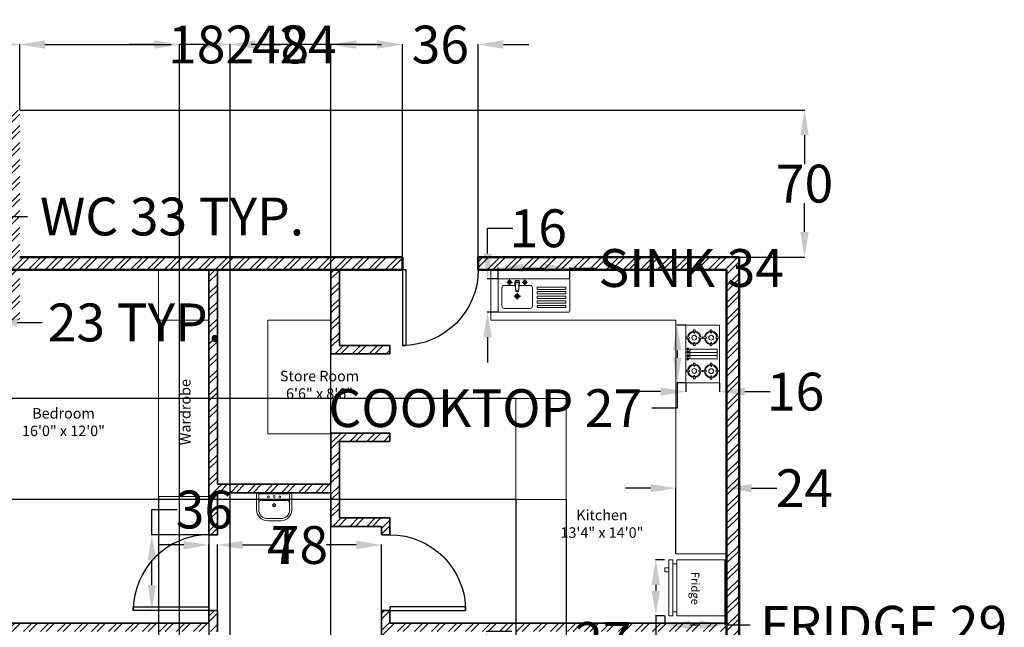
# Model space of a CAD drawing. Units: inches. Extents: x 7 to 752, y -275 to 426.
# Tile 5 of 5: x 284 to 752, y 137 to 426. Entities that reach past the tile are written whole.
import ezdxf

# ---------------------------------------------------------------- set-up
doc = ezdxf.new("R2010")
doc.units = ezdxf.units.IN
for name, color, linetype, lineweight in [('A-ANNO-DIMS', 2, 'Continuous', 18), ('A-ANNO-TEXT', 7, 'Continuous', 18), ('A-AREA-IDEN', 7, 'Continuous', 18), ('A-DOOR', 6, 'Continuous', 25), ('A-EQPM', 3, 'Continuous', 18), ('A-FLOR-CASE', 2, 'Continuous', 18), ('A-FLOR-FIXT', 8, 'Continuous', 18), ('A-WALL-PATT', 252, 'Continuous', 13), ('Inner Wall', 5, 'Continuous', 35), ('Kitchen', 3, 'Continuous', 18), ('Outer Wall', 1, 'Continuous', 50)]:
    doc.layers.add(name, color=color, linetype=linetype, lineweight=lineweight)
doc.styles.get("Standard").update_dxf_attribs({"font": 'arial.ttf'})
doc.dimstyles.get("Standard").update_dxf_attribs({"dimtxt": 18, "dimasz": 12, "dimexe": 0.18, "dimexo": 0.0625, "dimgap": 0.09, "dimtad": 0, "dimtih": 1, "dimtoh": 1, "dimdec": 0, "dimzin": 0, "dimdsep": 46, "dimlunit": 3, "dimtxsty": 'Standard', "dimcen": 0.09, "dimadec": 0, "dimazin": 0, "dimtfac": 1, "dimtdec": 0, "dimtofl": 0, "dimtmove": 0, "dimatfit": 3, "dimfxl": 1, "dimtolj": 1, "dimtzin": 0, "dimarcsym": 0})
pattern_1 = [(45, (-434.707, -1257.0093), (-4.041115, 4.041115), []), (45, (-432.013, -1257.0093), (-4.041115, 4.041115), [])]

# ---------------------------------------------------------------- blocks, each defined once
blk = doc.blocks.new('*U3')
for p, q in [((0, 0), (0, -4)), ((36, 0), (36, -4))]:
    blk.add_line(p, q)
blk.add_lwpolyline([(0, 0), (0, 36), (1.75, 36), (1.75, 0)], close=True)
blk.add_arc((0, 0), 36, 0, 90)
blk = doc.blocks.new('*U5')
for p, q in [((0, 0), (0, -6)), ((36, 0), (36, -6))]:
    blk.add_line(p, q)
blk.add_lwpolyline([(0, 0), (0, 36), (1.75, 36), (1.75, 0)], close=True)
blk.add_arc((0, 0), 36, 0, 90)
blk = doc.blocks.new('A$C7C492201')
for p, q in [((0, 10), (0, 427)), ((10, 437), (927, 437)), ((112, 389), (185, 389)), ((148, 425), (148, 352)), ((223, 415), (217, 376)), ((223, 415), (232, 268)), ((223, 415), (248, 415)), ((225, 395), (248, 395)), ((273, 415), (248, 415)), ((272, 395), (248, 395)), ((273, 415), (265, 268)), ((273, 415), (280, 376)), ((312, 389), (385, 389)), ((348, 425), (348, 352)), ((937, 10), (937, 427)), ((48, 319), (48, 79)), ((221, 349), (78, 349)), ((217, 376), (232, 268)), ((231, 279), (248, 279)), ((232, 268), (248, 268)), ((266, 279), (248, 279)), ((265, 268), (248, 268)), ((280, 376), (265, 268)), ((418, 349), (276, 349)), ((448, 319), (448, 79)), ((509, 328), (509, 298)), ((509, 328), (885, 328)), ((509, 298), (885, 298)), ((509, 268), (509, 238)), ((509, 268), (885, 268)), ((885, 328), (885, 298)), ((885, 268), (885, 238)), ((203, 208), (294, 208)), ((248, 253), (248, 163)), ((509, 238), (885, 238)), ((509, 208), (885, 208)), ((509, 208), (509, 178)), ((509, 178), (885, 178)), ((509, 148), (509, 118)), ((509, 148), (885, 148)), ((885, 208), (885, 178)), ((885, 148), (885, 118)), ((927, 0), (10, 0)), ((418, 49), (78, 49)), ((509, 118), (885, 118)), ((509, 88), (509, 58)), ((509, 88), (885, 88)), ((509, 58), (885, 58)), ((885, 88), (885, 58))]:
    blk.add_line(p, q)
for centre, radius in [((148, 389), 25), ((148, 389), 15), ((348, 389), 25), ((348, 389), 15), ((248, 208), 30), ((248, 208), 20)]:
    blk.add_circle(centre, radius)
for centre, radius, start, end in [((10, 427), 10, 90, 180), ((247, 388), 7.19, 80.5252, 279.4748), ((250, 388), 7.19, 260.5252, 99.4748), ((927, 427), 10, 0, 90), ((78, 319), 30, 90, 180), ((418, 319), 30, 0, 90), ((10, 10), 10, 180, 270), ((78, 79), 30, 180, 270), ((418, 79), 30, 270, 0), ((927, 10), 10, 270, 0)]:
    blk.add_arc(centre, radius, start, end)
blk = doc.blocks.new('REFRI-00')
for points in [[(-0.35, 0.35), (-0.35, -0.25), (0.35, -0.25), (0.35, 0.35), (-0.35, 0.35)], [(-0.35, -0.3), (-0.35, -0.35), (0.35, -0.35), (0.35, -0.3), (-0.35, -0.3)], [(-0.3, -0.3), (-0.3, -0.25)], [(-0.25, -0.35), (-0.25, -0.4), (-0.2, -0.4), (-0.2, -0.35)], [(0.3, -0.3), (0.3, -0.25)]]:
    blk.add_lwpolyline(points)
blk = doc.blocks.new('A$C57CF26DA')
for p, q in [((0, 0), (0, 420)), ((720, 420), (0, 420)), ((167, 413), (147, 413)), ((147, 413), (152, 373)), ((152, 373), (162, 373)), ((162, 373), (167, 413)), ((300, 391), (300, 49)), ((300, 391), (420, 391)), ((340, 391), (340, 49)), ((380, 391), (380, 49)), ((420, 391), (420, 49)), ((584, 413), (564, 413)), ((564, 413), (569, 373)), ((569, 373), (579, 373)), ((579, 373), (584, 413)), ((720, 0), (720, 420)), ((99, 320), (59, 325)), ((59, 325), (59, 305)), ((59, 305), (99, 310)), ((99, 310), (99, 320)), ((152, 257), (147, 217)), ((162, 257), (152, 257)), ((167, 217), (162, 257)), ((255, 325), (215, 320)), ((215, 320), (215, 310)), ((215, 310), (255, 305)), ((255, 305), (255, 325)), ((516, 320), (476, 325)), ((476, 325), (476, 305)), ((476, 305), (516, 310)), ((516, 310), (516, 320)), ((569, 257), (564, 217)), ((579, 257), (569, 257)), ((584, 217), (579, 257)), ((672, 325), (632, 320)), ((632, 320), (632, 310)), ((632, 310), (672, 305)), ((672, 305), (672, 325)), ((147, 217), (167, 217)), ((167, 203), (147, 203)), ((147, 203), (152, 163)), ((152, 163), (162, 163)), ((162, 163), (167, 203)), ((581, 203), (561, 203)), ((561, 203), (566, 163)), ((564, 217), (584, 217)), ((566, 163), (576, 163)), ((576, 163), (581, 203)), ((99, 110), (59, 115)), ((59, 115), (59, 95)), ((59, 95), (99, 100)), ((99, 100), (99, 110)), ((152, 47), (147, 7)), ((147, 7), (167, 7)), ((162, 47), (152, 47)), ((167, 7), (162, 47)), ((255, 115), (215, 110)), ((215, 110), (215, 100)), ((215, 100), (255, 95)), ((255, 95), (255, 115)), ((302, 39), (295, 39)), ((295, 39), (295, 11)), ((295, 11), (302, 11)), ((420, 49), (300, 49)), ((302, 11), (302, 39)), ((341, 39), (334, 39)), ((334, 39), (334, 11)), ((334, 11), (341, 11)), ((341, 11), (341, 39)), ((380, 11), (380, 39)), ((380, 39), (386, 39)), ((386, 11), (380, 11)), ((386, 39), (386, 11)), ((419, 11), (419, 39)), ((419, 39), (426, 39)), ((426, 11), (419, 11)), ((426, 39), (426, 11)), ((513, 110), (473, 115)), ((473, 115), (473, 95)), ((473, 95), (513, 100)), ((513, 100), (513, 110)), ((566, 47), (561, 7)), ((561, 7), (581, 7)), ((576, 47), (566, 47)), ((581, 7), (576, 47)), ((669, 115), (629, 110)), ((629, 110), (629, 100)), ((629, 100), (669, 95)), ((669, 95), (669, 115)), ((720, 0), (0, 0))]:
    blk.add_line(p, q)
for centre in [(157, 315), (574, 315), (157, 105), (571, 105)]:
    blk.add_circle(centre, 30)
for centre, radius, start, end in [((157, 315), 83, 95.5849, 174.4151), ((157, 315), 73, 95.3738, 174.6262), ((157, 315), 73, 5.3738, 84.6262), ((157, 315), 83, 5.5849, 84.4151), ((574, 315), 83, 95.5849, 174.4151), ((574, 315), 73, 95.3738, 174.6262), ((574, 315), 73, 5.3738, 84.6262), ((574, 315), 83, 5.5849, 84.4151), ((157, 315), 83, 185.5849, 264.4151), ((157, 315), 73, 185.3738, 264.6262), ((157, 315), 73, 275.3738, 354.6262), ((157, 315), 83, 275.5849, 354.4151), ((574, 315), 83, 185.5849, 264.4151), ((574, 315), 73, 185.3738, 264.6262), ((574, 315), 73, 275.3738, 354.6262), ((574, 315), 83, 275.5849, 354.4151), ((157, 105), 83, 95.5849, 174.4151), ((157, 105), 73, 95.3738, 174.6262), ((157, 105), 73, 5.3738, 84.6262), ((157, 105), 83, 5.5849, 84.4151), ((571, 105), 83, 95.5849, 174.4151), ((571, 105), 73, 95.3738, 174.6262), ((571, 105), 73, 5.3738, 84.6262), ((571, 105), 83, 5.5849, 84.4151), ((157, 105), 83, 185.5849, 264.4151), ((157, 105), 73, 185.3738, 264.6262), ((157, 105), 73, 275.3738, 354.6262), ((157, 105), 83, 275.5849, 354.4151), ((298, 25), 13.7, 104.4775, 255.5225), ((298, 25), 13.7, 284.4775, 75.5225), ((337, 25), 13.7, 104.4775, 255.5225), ((337, 25), 13.7, 284.4775, 75.5225), ((383, 25), 13.7, 104.4775, 255.5225), ((383, 25), 13.7, 284.4775, 75.5225), ((422, 25), 13.7, 104.4775, 255.5225), ((422, 25), 13.7, 284.4775, 75.5225), ((571, 105), 83, 185.5849, 264.4151), ((571, 105), 73, 185.3738, 264.6262), ((571, 105), 73, 275.3738, 354.6262), ((571, 105), 83, 275.5849, 354.4151)]:
    blk.add_arc(centre, radius, start, end)
blk = doc.blocks.new('A$C57EA129C')
for p, q in [((0, 0.443), (0, 0.178)), ((0.016, 0.459), (0.563, 0.459)), ((0.036, 0.432), (0.036, 0.29)), ((0.045, 0.441), (0.535, 0.441)), ((0.08, 0.334), (0.499, 0.334)), ((0.544, 0.432), (0.544, 0.29)), ((0.579, 0.443), (0.579, 0.178)), ((0.036, 0.29), (0.036, 0.178)), ((0.544, 0.29), (0.544, 0.178)), ((0.178, 0.036), (0.401, 0.036)), ((0.178, 0), (0.401, 0))]:
    blk.add_line(p, q)
for centre, radius in [((0.198, 0.392), 0.0143), ((0.29, 0.396), 0.0156), ((0.381, 0.392), 0.0143), ((0.29, 0.255), 0.0267), ((0.29, 0.255), 0.0178)]:
    blk.add_circle(centre, radius)
for centre, radius, start, end in [((0.016, 0.443), 0.016, 90, 180), ((0.045, 0.432), 0.00891, 90, 180), ((0.08, 0.29), 0.0445, 90, 180), ((0.499, 0.29), 0.0445, 0, 90), ((0.535, 0.432), 0.00891, 0, 90), ((0.563, 0.443), 0.016, 0, 90), ((0.178, 0.178), 0.178, 180, 270), ((0.178, 0.178), 0.143, 180, 270), ((0.401, 0.178), 0.178, 270, 0), ((0.401, 0.178), 0.143, 270, 0)]:
    blk.add_arc(centre, radius, start, end)
blk = doc.blocks.new('*D16')
at = {"layer": 'A-ANNO-DIMS', "color": 0, "lineweight": -2, "transparency": 16777216}
for p, q in [((276.06, 320.03), (276.06, 332.03)), ((276.06, 332.03), (288.06, 332.03)), ((271.12, 320.03), (276.24, 320.03)), ((276.06, 298.68), (276.06, 308.03)), ((271.12, 286.68), (276.24, 286.68))]:
    blk.add_line(p, q, dxfattribs=at)
at = {"layer": 'A-ANNO-DIMS', "color": 0, "transparency": 16777216}
for points in [[(274.06, 308.03), (278.06, 308.03), (276.06, 320.03)], [(274.06, 298.68), (278.06, 298.68), (276.06, 286.68)]]:
    blk.add_solid(points, dxfattribs=at)
at = {"layer": 'Defpoints', "color": 0, "transparency": 16777216}
for p in [(271.06, 320.03), (276.06, 320.03), (271.06, 286.68)]:
    blk.add_point(p, dxfattribs=at)
at = {"layer": 'A-ANNO-DIMS', "color": 0, "transparency": 16777216, "insert": (356.77, 332.03), "char_height": 18, "attachment_point": 5}
blk.add_mtext('\\A1;WC 33 TYP.', dxfattribs=at)
blk = doc.blocks.new('*D17')
at = {"layer": 'A-ANNO-DIMS', "color": 0, "lineweight": -2, "transparency": 16777216}
for p, q in [((247.6, 286.61), (247.6, 281.49)), ((271.06, 286.61), (271.06, 281.49)), ((235.6, 281.67), (223.6, 281.67)), ((283.06, 281.67), (295.06, 281.67))]:
    blk.add_line(p, q, dxfattribs=at)
at = {"layer": 'A-ANNO-DIMS', "color": 0, "transparency": 16777216}
for points in [[(235.6, 283.67), (235.6, 279.67), (247.6, 281.67)], [(283.06, 283.67), (283.06, 279.67), (271.06, 281.67)]]:
    blk.add_solid(points, dxfattribs=at)
at = {"layer": 'Defpoints', "color": 0, "transparency": 16777216}
for p in [(247.6, 286.68), (271.06, 286.68), (271.06, 281.67)]:
    blk.add_point(p, dxfattribs=at)
at = {"layer": 'A-ANNO-DIMS', "color": 0, "transparency": 16777216, "insert": (339.11, 281.67), "char_height": 18, "attachment_point": 5}
blk.add_mtext('\\A1;23 TYP.', dxfattribs=at)
blk = doc.blocks.new('*D20')
at = {"layer": 'A-ANNO-DIMS', "color": 0, "lineweight": -2, "transparency": 16777216}
for p, q in [((518.33, 134.68), (506.15, 134.68)), ((506.33, 122.68), (506.33, 103.84)), ((506.33, 66.2), (506.33, 85.04)), ((518.33, 54.2), (506.15, 54.2))]:
    blk.add_line(p, q, dxfattribs=at)
at = {"layer": 'A-ANNO-DIMS', "color": 0, "transparency": 16777216}
for points in [[(504.33, 122.68), (508.33, 122.68), (506.33, 134.68)], [(504.33, 66.2), (508.33, 66.2), (506.33, 54.2)]]:
    blk.add_solid(points, dxfattribs=at)
at = {"layer": 'Defpoints', "color": 0, "transparency": 16777216}
for p in [(506.33, 134.68), (518.4, 134.68), (518.4, 54.2)]:
    blk.add_point(p, dxfattribs=at)
at = {"layer": 'A-ANNO-DIMS', "color": 0, "transparency": 16777216, "insert": (506.33, 94.44), "char_height": 18, "attachment_point": 5}
blk.add_mtext('\\A1;KING BED 80 TYP.', dxfattribs=at)
blk = doc.blocks.new('*D24')
at = {"layer": 'A-ANNO-DIMS', "color": 0, "lineweight": -2, "transparency": 16777216}
for p, q in [((511.85, 302.5), (511.85, 307.72)), ((523.85, 307.54), (533.86, 307.54)), ((545.86, 302.5), (545.86, 307.72)), ((545.86, 307.54), (557.86, 307.54))]:
    blk.add_line(p, q, dxfattribs=at)
at = {"layer": 'A-ANNO-DIMS', "color": 0, "transparency": 16777216}
for points in [[(523.85, 309.54), (523.85, 305.54), (511.85, 307.54)], [(533.86, 309.54), (533.86, 305.54), (545.86, 307.54)]]:
    blk.add_solid(points, dxfattribs=at)
at = {"layer": 'Defpoints', "color": 0, "transparency": 16777216}
for p in [(545.86, 307.54), (511.85, 302.44), (545.86, 302.44)]:
    blk.add_point(p, dxfattribs=at)
at = {"layer": 'A-ANNO-DIMS', "color": 0, "transparency": 16777216, "insert": (603.6, 307.54), "char_height": 18, "attachment_point": 5}
blk.add_mtext('\\A1;SINK 34', dxfattribs=at)
blk = doc.blocks.new('*D25')
at = {"layer": 'A-ANNO-DIMS', "color": 0, "lineweight": -2, "transparency": 16777216}
for p, q in [((506.75, 314.44), (506.75, 326.44)), ((506.75, 326.44), (518.75, 326.44)), ((511.79, 302.44), (506.57, 302.44)), ((511.79, 286.59), (506.57, 286.59)), ((506.75, 274.59), (506.75, 262.59))]:
    blk.add_line(p, q, dxfattribs=at)
at = {"layer": 'A-ANNO-DIMS', "color": 0, "transparency": 16777216}
for points in [[(504.75, 314.44), (508.75, 314.44), (506.75, 302.44)], [(504.75, 274.59), (508.75, 274.59), (506.75, 286.59)]]:
    blk.add_solid(points, dxfattribs=at)
at = {"layer": 'Defpoints', "color": 0, "transparency": 16777216}
for p in [(506.75, 302.44), (511.85, 302.44), (511.85, 286.59)]:
    blk.add_point(p, dxfattribs=at)
at = {"layer": 'A-ANNO-DIMS', "color": 0, "transparency": 16777216, "insert": (530.88, 326.44), "char_height": 18, "attachment_point": 5}
blk.add_mtext('\\A1;16', dxfattribs=at)
blk = doc.blocks.new('*D26')
at = {"layer": 'A-ANNO-DIMS', "color": 0, "lineweight": -2, "transparency": 16777216}
for p, q in [((591.04, 142.1), (591.04, 137.69)), ((619.61, 142.1), (619.61, 137.69)), ((603.04, 137.87), (607.61, 137.87)), ((619.61, 137.87), (631.61, 137.87))]:
    blk.add_line(p, q, dxfattribs=at)
at = {"layer": 'A-ANNO-DIMS', "color": 0, "transparency": 16777216}
for points in [[(603.04, 139.87), (603.04, 135.87), (591.04, 137.87)], [(607.61, 139.87), (607.61, 135.87), (619.61, 137.87)]]:
    blk.add_solid(points, dxfattribs=at)
at = {"layer": 'Defpoints', "color": 0, "transparency": 16777216}
for p in [(591.04, 142.16), (619.61, 142.16), (619.61, 137.87)]:
    blk.add_point(p, dxfattribs=at)
at = {"layer": 'A-ANNO-DIMS', "color": 0, "transparency": 16777216, "insert": (695.1, 137.87), "char_height": 18, "attachment_point": 5}
blk.add_mtext('\\A1;FRIDGE 29', dxfattribs=at)
blk = doc.blocks.new('*D27')
at = {"layer": 'A-ANNO-DIMS', "color": 0, "lineweight": -2, "transparency": 16777216}
for p, q in [((590.98, 168.83), (586.58, 168.83)), ((586.76, 156.83), (586.76, 154.16)), ((590.98, 142.16), (586.58, 142.16)), ((586.76, 142.16), (586.76, 130.16)), ((586.76, 130.16), (574.76, 130.16))]:
    blk.add_line(p, q, dxfattribs=at)
at = {"layer": 'A-ANNO-DIMS', "color": 0, "transparency": 16777216}
for points in [[(584.76, 156.83), (588.76, 156.83), (586.76, 168.83)], [(584.76, 154.16), (588.76, 154.16), (586.76, 142.16)]]:
    blk.add_solid(points, dxfattribs=at)
at = {"layer": 'Defpoints', "color": 0, "transparency": 16777216}
for p in [(591.04, 168.83), (586.76, 142.16), (591.04, 142.16)]:
    blk.add_point(p, dxfattribs=at)
at = {"layer": 'A-ANNO-DIMS', "color": 0, "transparency": 16777216, "insert": (561.62, 130.16), "char_height": 18, "attachment_point": 5}
blk.add_mtext('\\A1;27', dxfattribs=at)
blk = doc.blocks.new('*D28')
at = {"layer": 'A-ANNO-DIMS', "color": 0, "lineweight": -2, "transparency": 16777216}
for p, q in [((600.98, 280.39), (596.74, 280.39)), ((596.92, 268.39), (596.92, 264.9)), ((600.98, 252.9), (596.74, 252.9)), ((596.92, 252.9), (596.92, 240.9)), ((596.92, 240.9), (584.92, 240.9))]:
    blk.add_line(p, q, dxfattribs=at)
at = {"layer": 'A-ANNO-DIMS', "color": 0, "transparency": 16777216}
for points in [[(594.92, 268.39), (598.92, 268.39), (596.92, 280.39)], [(594.92, 264.9), (598.92, 264.9), (596.92, 252.9)]]:
    blk.add_solid(points, dxfattribs=at)
at = {"layer": 'Defpoints', "color": 0, "transparency": 16777216}
for p in [(601.05, 280.39), (596.92, 252.9), (601.05, 252.9)]:
    blk.add_point(p, dxfattribs=at)
at = {"layer": 'A-ANNO-DIMS', "color": 0, "transparency": 16777216, "insert": (505.68, 240.9), "char_height": 18, "attachment_point": 5}
blk.add_mtext('\\A1;COOKTOP 27', dxfattribs=at)
blk = doc.blocks.new('*D29')
at = {"layer": 'A-ANNO-DIMS', "color": 0, "lineweight": -2, "transparency": 16777216}
for p, q in [((601.05, 252.84), (601.05, 248.6)), ((617.08, 252.84), (617.08, 248.6)), ((589.05, 248.78), (577.05, 248.78)), ((629.08, 248.78), (641.08, 248.78))]:
    blk.add_line(p, q, dxfattribs=at)
at = {"layer": 'A-ANNO-DIMS', "color": 0, "transparency": 16777216}
for points in [[(589.05, 250.78), (589.05, 246.78), (601.05, 248.78)], [(629.08, 250.78), (629.08, 246.78), (617.08, 248.78)]]:
    blk.add_solid(points, dxfattribs=at)
at = {"layer": 'Defpoints', "color": 0, "transparency": 16777216}
for p in [(601.05, 252.9), (617.08, 252.9), (617.08, 248.78)]:
    blk.add_point(p, dxfattribs=at)
at = {"layer": 'A-ANNO-DIMS', "color": 0, "transparency": 16777216, "insert": (653.21, 248.78), "char_height": 18, "attachment_point": 5}
blk.add_mtext('\\A1;16', dxfattribs=at)
blk = doc.blocks.new('*D33')
at = {"layer": 'A-ANNO-DIMS', "color": 0, "lineweight": -2, "transparency": 16777216}
for p, q in [((176.33, 382.74), (176.33, 414.01)), ((188.33, 413.83), (211.18, 413.83)), ((272.33, 413.83), (249.47, 413.83)), ((284.33, 382.74), (284.33, 414.01))]:
    blk.add_line(p, q, dxfattribs=at)
at = {"layer": 'A-ANNO-DIMS', "color": 0, "transparency": 16777216}
for points in [[(188.33, 415.83), (188.33, 411.83), (176.33, 413.83)], [(272.33, 415.83), (272.33, 411.83), (284.33, 413.83)]]:
    blk.add_solid(points, dxfattribs=at)
at = {"layer": 'Defpoints', "color": 0, "transparency": 16777216}
for p in [(284.33, 413.83), (176.33, 382.68), (284.33, 382.68)]:
    blk.add_point(p, dxfattribs=at)
at = {"layer": 'A-ANNO-DIMS', "color": 0, "transparency": 16777216, "insert": (230.33, 413.83), "char_height": 18, "attachment_point": 5}
blk.add_mtext('\\A1;108', dxfattribs=at)
blk = doc.blocks.new('*D34')
at = {"layer": 'A-ANNO-DIMS', "color": 0, "lineweight": -2, "transparency": 16777216}
for p, q in [((284.33, 382.74), (284.33, 414.01)), ((296.33, 413.83), (356.29, 413.83)), ((454.33, 413.83), (394.36, 413.83)), ((466.33, 312.74), (466.33, 414.01))]:
    blk.add_line(p, q, dxfattribs=at)
at = {"layer": 'A-ANNO-DIMS', "color": 0, "transparency": 16777216}
for points in [[(296.33, 415.83), (296.33, 411.83), (284.33, 413.83)], [(454.33, 415.83), (454.33, 411.83), (466.33, 413.83)]]:
    blk.add_solid(points, dxfattribs=at)
at = {"layer": 'Defpoints', "color": 0, "transparency": 16777216}
for p in [(466.33, 413.83), (284.33, 382.68), (466.33, 312.68)]:
    blk.add_point(p, dxfattribs=at)
at = {"layer": 'A-ANNO-DIMS', "color": 0, "transparency": 16777216, "insert": (375.33, 413.83), "char_height": 18, "attachment_point": 5}
blk.add_mtext('\\A1;182', dxfattribs=at)
blk = doc.blocks.new('*D35')
at = {"layer": 'A-ANNO-DIMS', "color": 0, "lineweight": -2, "transparency": 16777216}
for p, q in [((454.328243, 413.826615), (442.328243, 413.826615)), ((466.328243, 312.739115), (466.328243, 414.006615)), ((502.328243, 312.739115), (502.328243, 414.006615)), ((514.328243, 413.826615), (526.328243, 413.826615))]:
    blk.add_line(p, q, dxfattribs=at)
at = {"layer": 'A-ANNO-DIMS', "color": 0, "transparency": 16777216}
for points in [[(454.328243, 415.826615), (454.328243, 411.826615), (466.328243, 413.826615)], [(514.328243, 415.826615), (514.328243, 411.826615), (502.328243, 413.826615)]]:
    blk.add_solid(points, dxfattribs=at)
at = {"layer": 'Defpoints', "color": 0, "transparency": 16777216}
for p in [(502.328243, 413.826615), (466.328243, 312.676615), (502.328243, 312.676615)]:
    blk.add_point(p, dxfattribs=at)
at = {"layer": 'A-ANNO-DIMS', "color": 0, "transparency": 16777216, "insert": (484.328243, 413.826615), "char_height": 18, "attachment_point": 5}
blk.add_mtext('\\A1;36', dxfattribs=at)
blk = doc.blocks.new('*D36')
at = {"layer": 'A-ANNO-DIMS', "color": 0, "lineweight": -2, "transparency": 16777216}
for p, q in [((284.39, 382.68), (657.66, 382.68)), ((657.48, 370.68), (657.48, 356.96)), ((657.48, 324.68), (657.48, 338.4)), ((626.39, 312.68), (657.66, 312.68))]:
    blk.add_line(p, q, dxfattribs=at)
at = {"layer": 'A-ANNO-DIMS', "color": 0, "transparency": 16777216}
for points in [[(655.48, 370.68), (659.48, 370.68), (657.48, 382.68)], [(655.48, 324.68), (659.48, 324.68), (657.48, 312.68)]]:
    blk.add_solid(points, dxfattribs=at)
at = {"layer": 'Defpoints', "color": 0, "transparency": 16777216}
for p in [(284.33, 382.68), (626.33, 312.68), (657.48, 312.68)]:
    blk.add_point(p, dxfattribs=at)
at = {"layer": 'A-ANNO-DIMS', "color": 0, "transparency": 16777216, "insert": (657.48, 347.68), "char_height": 18, "attachment_point": 5}
blk.add_mtext('\\A1;70', dxfattribs=at)
blk = doc.blocks.new('*D39')
at = {"layer": 'A-ANNO-DIMS', "color": 0, "lineweight": -2, "transparency": 16777216}
for p, q in [((348.33, 413.83), (336.33, 413.83)), ((360.33, -131.26), (360.33, 414.01)), ((384.33, -131.26), (384.33, 414.01)), ((396.33, 413.83), (408.33, 413.83))]:
    blk.add_line(p, q, dxfattribs=at)
at = {"layer": 'A-ANNO-DIMS', "color": 0, "transparency": 16777216}
for points in [[(348.33, 415.83), (348.33, 411.83), (360.33, 413.83)], [(396.33, 415.83), (396.33, 411.83), (384.33, 413.83)]]:
    blk.add_solid(points, dxfattribs=at)
at = {"layer": 'Defpoints', "color": 0, "transparency": 16777216}
for p in [(384.33, 413.83), (360.33, -131.32), (384.33, -131.32)]:
    blk.add_point(p, dxfattribs=at)
at = {"layer": 'A-ANNO-DIMS', "color": 0, "transparency": 16777216, "insert": (421.43, 413.83), "char_height": 18, "attachment_point": 5}
blk.add_mtext('\\A1;24', dxfattribs=at)
blk = doc.blocks.new('*D40')
at = {"layer": 'A-ANNO-DIMS', "color": 0, "lineweight": -2, "transparency": 16777216}
for p, q in [((372.328243, 413.826615), (360.328243, 413.826615)), ((384.328243, -106.961989), (384.328243, 414.006615)), ((432.328243, -106.961989), (432.328243, 414.006615)), ((444.328243, 413.826615), (456.328243, 413.826615))]:
    blk.add_line(p, q, dxfattribs=at)
at = {"layer": 'A-ANNO-DIMS', "color": 0, "transparency": 16777216}
for points in [[(372.328243, 415.826615), (372.328243, 411.826615), (384.328243, 413.826615)], [(444.328243, 415.826615), (444.328243, 411.826615), (432.328243, 413.826615)]]:
    blk.add_solid(points, dxfattribs=at)
at = {"layer": 'Defpoints', "color": 0, "transparency": 16777216}
for p in [(432.328243, 413.826615), (384.328243, -107.024489), (432.328243, -107.024489)]:
    blk.add_point(p, dxfattribs=at)
at = {"layer": 'A-ANNO-DIMS', "color": 0, "transparency": 16777216, "insert": (408.328243, 413.826615), "char_height": 18, "attachment_point": 5}
blk.add_mtext('\\A1;48', dxfattribs=at)
blk = doc.blocks.new('*D46')
at = {"layer": 'A-ANNO-DIMS', "color": 0, "lineweight": -2, "transparency": 16777216}
for p, q in [((520.16, 197.44), (520.16, -259.65)), ((544.16, 197.44), (544.16, -259.65)), ((508.16, -259.47), (496.16, -259.47)), ((556.16, -259.47), (568.16, -259.47))]:
    blk.add_line(p, q, dxfattribs=at)
at = {"layer": 'A-ANNO-DIMS', "color": 0, "transparency": 16777216}
for points in [[(508.16, -257.47), (508.16, -261.47), (520.16, -259.47)], [(556.16, -257.47), (556.16, -261.47), (544.16, -259.47)]]:
    blk.add_solid(points, dxfattribs=at)
at = {"layer": 'Defpoints', "color": 0, "transparency": 16777216}
for p in [(520.16, 197.5), (544.16, 197.5), (544.16, -259.47)]:
    blk.add_point(p, dxfattribs=at)
at = {"layer": 'A-ANNO-DIMS', "color": 0, "transparency": 16777216, "insert": (581.26, -259.47), "char_height": 18, "attachment_point": 5}
blk.add_mtext('\\A1;24', dxfattribs=at)
blk = doc.blocks.new('*D47')
at = {"layer": 'A-ANNO-DIMS', "color": 0, "lineweight": -2, "transparency": 16777216}
for p, q in [((520.1, 245.5), (127, 245.5)), ((127.18, 233.5), (127.18, 230.78)), ((127.18, 209.5), (127.18, 212.22)), ((520.1, 197.5), (127, 197.5))]:
    blk.add_line(p, q, dxfattribs=at)
at = {"layer": 'A-ANNO-DIMS', "color": 0, "transparency": 16777216}
for points in [[(125.18, 233.5), (129.18, 233.5), (127.18, 245.5)], [(125.18, 209.5), (129.18, 209.5), (127.18, 197.5)]]:
    blk.add_solid(points, dxfattribs=at)
at = {"layer": 'Defpoints', "color": 0, "transparency": 16777216}
for p in [(127.18, 245.5), (520.16, 245.5), (520.16, 197.5)]:
    blk.add_point(p, dxfattribs=at)
at = {"layer": 'A-ANNO-DIMS', "color": 0, "transparency": 16777216, "insert": (127.18, 221.5), "char_height": 18, "attachment_point": 5}
blk.add_mtext('\\A1;48', dxfattribs=at)
blk = doc.blocks.new('*D48')
at = {"layer": 'A-ANNO-DIMS', "color": 0, "lineweight": -2, "transparency": 16777216}
for p, q in [((584.33, 202.83), (572.33, 202.83)), ((596.33, 171.74), (596.33, 203.01)), ((620.33, 171.74), (620.33, 203.01)), ((632.33, 202.83), (644.33, 202.83))]:
    blk.add_line(p, q, dxfattribs=at)
at = {"layer": 'A-ANNO-DIMS', "color": 0, "transparency": 16777216}
for points in [[(584.33, 204.83), (584.33, 200.83), (596.33, 202.83)], [(632.33, 204.83), (632.33, 200.83), (620.33, 202.83)]]:
    blk.add_solid(points, dxfattribs=at)
at = {"layer": 'Defpoints', "color": 0, "transparency": 16777216}
for p in [(620.33, 202.83), (596.33, 171.68), (620.33, 171.68)]:
    blk.add_point(p, dxfattribs=at)
at = {"layer": 'A-ANNO-DIMS', "color": 0, "transparency": 16777216, "insert": (657.43, 202.83), "char_height": 18, "attachment_point": 5}
blk.add_mtext('\\A1;24', dxfattribs=at)
blk = doc.blocks.new('*D50')
at = {"layer": 'A-ANNO-DIMS', "color": 0, "lineweight": -2, "transparency": 16777216}
for p, q in [((362.33, 175.83), (350.33, 175.83)), ((374.33, 144.74), (374.33, 176.01)), ((378.33, 144.74), (378.33, 176.01)), ((390.33, 175.83), (402.33, 175.83))]:
    blk.add_line(p, q, dxfattribs=at)
at = {"layer": 'A-ANNO-DIMS', "color": 0, "transparency": 16777216}
for points in [[(362.33, 177.83), (362.33, 173.83), (374.33, 175.83)], [(390.33, 177.83), (390.33, 173.83), (378.33, 175.83)]]:
    blk.add_solid(points, dxfattribs=at)
at = {"layer": 'Defpoints', "color": 0, "transparency": 16777216}
for p in [(378.33, 175.83), (374.33, 144.68), (378.33, 144.68)]:
    blk.add_point(p, dxfattribs=at)
at = {"layer": 'A-ANNO-DIMS', "color": 0, "transparency": 16777216, "insert": (408.64, 175.83), "char_height": 18, "attachment_point": 5}
blk.add_mtext('\\A1;4', dxfattribs=at)
blk = doc.blocks.new('*D52')
at = {"layer": 'A-ANNO-DIMS', "color": 0, "lineweight": -2, "transparency": 16777216}
for p, q in [((350.33, 198.78), (350.33, -259.65)), ((374.33, 198.78), (374.33, -259.65)), ((338.33, -259.47), (326.33, -259.47)), ((386.33, -259.47), (398.33, -259.47))]:
    blk.add_line(p, q, dxfattribs=at)
at = {"layer": 'A-ANNO-DIMS', "color": 0, "transparency": 16777216}
for points in [[(338.33, -257.47), (338.33, -261.47), (350.33, -259.47)], [(386.33, -257.47), (386.33, -261.47), (374.33, -259.47)]]:
    blk.add_solid(points, dxfattribs=at)
at = {"layer": 'Defpoints', "color": 0, "transparency": 16777216}
for p in [(350.33, 198.85), (374.33, 198.85), (374.33, -259.47)]:
    blk.add_point(p, dxfattribs=at)
at = {"layer": 'A-ANNO-DIMS', "color": 0, "transparency": 16777216, "insert": (411.43, -259.47), "char_height": 18, "attachment_point": 5}
blk.add_mtext('\\A1;24', dxfattribs=at)
blk = doc.blocks.new('*D53')
at = {"layer": 'A-ANNO-DIMS', "color": 0, "lineweight": -2, "transparency": 16777216}
for p, q in [((378.33, 144.74), (378.33, 176.01)), ((390.33, 175.83), (404.4, 175.83)), ((444.33, 175.83), (430.26, 175.83)), ((456.33, 144.74), (456.33, 176.01))]:
    blk.add_line(p, q, dxfattribs=at)
at = {"layer": 'A-ANNO-DIMS', "color": 0, "transparency": 16777216}
for points in [[(390.33, 177.83), (390.33, 173.83), (378.33, 175.83)], [(444.33, 177.83), (444.33, 173.83), (456.33, 175.83)]]:
    blk.add_solid(points, dxfattribs=at)
at = {"layer": 'Defpoints', "color": 0, "transparency": 16777216}
for p in [(456.33, 175.83), (378.33, 144.68), (456.33, 144.68)]:
    blk.add_point(p, dxfattribs=at)
at = {"layer": 'A-ANNO-DIMS', "color": 0, "transparency": 16777216, "insert": (417.33, 175.83), "char_height": 18, "attachment_point": 5}
blk.add_mtext('\\A1;78', dxfattribs=at)
blk = doc.blocks.new('*D54')
at = {"layer": 'A-ANNO-DIMS', "color": 0, "lineweight": -2, "transparency": 16777216}
for p, q in [((347.18, 180.68), (347.18, 192.68)), ((347.18, 192.68), (359.18, 192.68)), ((378.27, 180.68), (347, 180.68)), ((347.18, 156.68), (347.18, 168.68)), ((378.27, 144.68), (347, 144.68))]:
    blk.add_line(p, q, dxfattribs=at)
at = {"layer": 'A-ANNO-DIMS', "color": 0, "transparency": 16777216}
for points in [[(345.18, 168.68), (349.18, 168.68), (347.18, 180.68)], [(345.18, 156.68), (349.18, 156.68), (347.18, 144.68)]]:
    blk.add_solid(points, dxfattribs=at)
at = {"layer": 'Defpoints', "color": 0, "transparency": 16777216}
for p in [(347.18, 180.68), (378.33, 180.68), (378.33, 144.68)]:
    blk.add_point(p, dxfattribs=at)
at = {"layer": 'A-ANNO-DIMS', "color": 0, "transparency": 16777216, "insert": (372.15, 192.68), "char_height": 18, "attachment_point": 5}
blk.add_mtext('\\A1;36', dxfattribs=at)

msp = doc.modelspace()

# ---------------------------------------------------------------- hatches: boundary and pattern name
at = {"layer": 'A-WALL-PATT'}
h = msp.add_hatch(dxfattribs=at)
h.set_pattern_fill('ANSI32', color=256, scale=0.6)
h.set_pattern_definition(pattern_1)
h.paths.add_polyline_path([(182.33, 376.68), (278.33, 376.68), (278.33, 306.68), (466.33, 306.68), (466.33, 312.68), (284.33, 312.68), (284.33, 382.68), (176.33, 382.68), (176.33, -48.32), (158.33, -48.32), (158.33, -228.32), (360.33, -228.32), (360.33, -137.32), (384.33, -137.32), (384.33, -131.32), (356.33, -131.32), (356.33, -222.32), (164.33, -222.32), (164.33, -54.32), (182.33, -54.32)])
h.paths.add_polyline_path([(626.33, 312.68), (502.33, 312.68), (502.33, 306.68), (620.33, 306.68), (620.33, 171.68), (620.33, -48.32), (544.33, -48.32), (544.33, -131.32), (432.33, -131.32), (432.33, -137.32), (550.33, -137.32), (550.33, -52.32), (626.33, -52.32)])
h = msp.add_hatch(dxfattribs=at)
h.set_pattern_fill('ANSI32', color=256, scale=0.6)
h.set_pattern_definition(pattern_1)
h.paths.add_polyline_path([(360.33, -48.32), (282.33, -48.32), (282.33, -44.32), (278.33, -44.32), (278.33, -48.32), (182.33, -48.32), (182.33, -54.32), (356.33, -54.32), (356.33, -89.32), (360.33, -89.32)])
h.paths.add_polyline_path([(484.33, -48.32), (460.33, -48.32), (460.33, -42.32), (456.33, -42.32), (456.33, -48.32), (432.33, -48.32), (432.33, -52.32), (456.33, -52.32), (456.33, -131.32), (460.33, -131.32), (460.33, -52.32), (484.33, -52.32)])
h.paths.add_polyline_path([(544.33, -48.32), (512.33, -48.32), (512.33, -52.32), (544.33, -52.32)])
h.paths.add_polyline_path([(460.33, 134.68), (484.33, 134.68), (620.33, 134.68), (620.33, 138.68), (460.33, 138.68), (460.33, 144.68), (456.33, 144.68), (456.33, -6.32), (460.33, -6.32)])
h.paths.add_polyline_path([(282.33, 3.68), (182.33, 3.68), (182.33, -0.32), (278.33, -0.32), (278.33, -16.32), (282.33, -16.32)])
h.paths.add_polyline_path([(378.33, 144.68), (374.33, 144.68), (374.33, 138.68), (182.33, 138.68), (182.33, 134.68), (378.33, 134.68)])
h.paths.add_polyline_path([(284.33, 306.68), (278.33, 306.68), (278.33, 286.68), (240.33, 286.68), (240.33, 282.68), (284.33, 282.68)])
h.paths.add_polyline_path([(212.33, 286.68), (182.33, 286.68), (182.33, 282.68), (212.33, 282.68)])
h.paths.add_polyline_path([(436.33, 225.08), (460.33, 225.08), (460.33, 229.08), (432.33, 229.08), (432.33, 184.68), (456.33, 184.68), (456.33, 180.68), (460.33, 180.68), (460.33, 188.68), (436.33, 188.68)])
h.paths.add_polyline_path([(432.33, 204.68), (378.33, 204.68), (378.33, 306.68), (374.33, 306.68), (374.33, 282.68), (374.33, 198.85), (374.33, 180.68), (378.33, 180.68), (378.33, 200.68), (432.33, 200.68)])
h.paths.add_polyline_path([(460.33, 270.68), (436.33, 270.68), (436.33, 306.68), (432.33, 306.68), (432.33, 282.68), (432.33, 266.68), (460.33, 266.68)])

# ---------------------------------------------------------------- linework, layer by layer
at = {"layer": 'A-FLOR-CASE'}
for points in [[(350.33, 306.68), (374.33, 306.68), (374.33, 282.68), (350.33, 282.68)], [(402.33, 282.68), (432.33, 282.68), (432.33, 306.68), (378.33, 306.68), (378.33, 204.68), (432.33, 204.68), (432.33, 228.68), (402.33, 228.68)], [(374.33, 282.68), (350.33, 282.68), (350.33, 198.85), (374.33, 198.85)]]:
    msp.add_lwpolyline(points, close=True, dxfattribs=at)
at = {"layer": 'Inner Wall'}
for p, q in [((374.33, 306.68), (374.33, 180.68)), ((378.33, 306.68), (378.33, 204.68)), ((432.33, 306.68), (432.33, 266.68)), ((436.33, 306.68), (436.33, 270.68)), ((436.33, 270.68), (460.33, 270.68)), ((460.33, 270.68), (460.33, 266.68)), ((432.33, 266.68), (460.33, 266.68)), ((432.33, 229.08), (460.33, 229.08)), ((432.33, 229.08), (432.33, 204.68)), ((436.33, 225.08), (460.33, 225.08)), ((436.33, 225.08), (436.33, 188.68)), ((460.33, 229.08), (460.33, 225.08)), ((378.33, 204.68), (432.33, 204.68)), ((378.33, 200.68), (432.33, 200.68)), ((378.33, 200.68), (378.33, 180.68)), ((432.33, 200.68), (432.33, 184.68)), ((436.33, 188.68), (460.33, 188.68)), ((460.33, 188.68), (460.33, 180.68)), ((432.33, 184.68), (456.33, 184.68)), ((456.33, 184.68), (456.33, 180.68)), ((374.33, 180.68), (378.33, 180.68)), ((460.33, 180.68), (456.33, 180.68)), ((374.33, 144.68), (378.33, 144.68)), ((374.33, 144.68), (374.33, 138.68)), ((378.33, 144.68), (378.33, 134.68)), ((460.33, 144.68), (456.33, 144.68)), ((456.33, 144.68), (456.33, -6.32)), ((460.33, 144.68), (460.33, 138.68)), ((182.33, 138.68), (374.33, 138.68)), ((460.33, 138.68), (620.33, 138.68))]:
    msp.add_line(p, q, dxfattribs=at)
at = {"layer": 'Kitchen'}
for points in [[(508.33, 306.68), (620.33, 306.68), (620.33, 171.68), (596.33, 171.68), (596.33, 282.68), (508.33, 282.68)], [(520.16, 245.5), (544.16, 245.5), (544.16, 197.5), (520.16, 197.5)]]:
    msp.add_lwpolyline(points, close=True, dxfattribs=at)
at = {"layer": 'Outer Wall'}
for p, q in [((466.33, 312.68), (284.33, 312.68)), ((466.33, 312.68), (466.33, 306.68)), ((626.33, 312.68), (502.33, 312.68)), ((502.33, 312.68), (502.33, 306.68)), ((626.33, -52.32), (626.33, 312.68)), ((278.33, 306.68), (466.33, 306.68)), ((502.33, 306.68), (620.33, 306.68)), ((620.33, -48.32), (620.33, 306.68))]:
    msp.add_line(p, q, dxfattribs=at)

# ---------------------------------------------------------------- block references
at = {"layer": 'A-DOOR', "xscale": -1}
for name, p, rotation in [('*U5', (466.33, 306.68), 180), ('*U3', (460.33, 144.68), 270)]:
    msp.add_blockref(name, p, dxfattribs=dict(at, rotation=rotation))
at = {"layer": 'A-DOOR', "rotation": 90}
msp.add_blockref('*U3', (374.33, 144.68), dxfattribs=at)
at = {"layer": 'A-EQPM'}
for name, p, xscale, yscale, zscale, rotation in [('A$C57CF26DA', (601.05, 280.39), 0.0381707681172169, 0.0381707681172169, 0.0381707681172169, 270), ('REFRI-00', (606.28, 155.49), 38.0932829071003, 38.0932829071003, 38.0932829071003, 269.9999999999999)]:
    msp.add_blockref(name, p, dxfattribs=dict(at, xscale=xscale, yscale=yscale, zscale=zscale, rotation=rotation))
at = {"layer": 'A-FLOR-FIXT'}
for name, p, xscale, yscale, zscale in [('A$C7C492201', (511.85, 286.59), 0.0362851414289068, 0.0362851414289068, 0.0362851414289068), ('A$C57EA129C', (413.72, 187.38), -28.98333223671166, 28.98333223671166, 28.98333223671166)]:
    msp.add_blockref(name, p, dxfattribs=dict(at, xscale=xscale, yscale=yscale, zscale=zscale))

# ---------------------------------------------------------------- texts
at = {"layer": 'A-ANNO-TEXT'}
for s, width, gutter_width, insert, char_height, attachment_point, rotation in [('\\pxqc;{\\fTimes New Roman|b0|i0|c0|p18;Wardrobe}', 49.1019, 12.5, (360.55, 263.54), 5, 3, 90), ('\\pxqc;{\\fTimes New Roman|b0|i0|c0|p18;Fridge}', 17.9518, 4.85, (607.46, 164.17), 3.878, 1, 270)]:
    msp.add_mtext_dynamic_manual_height_columns(s, width=width, gutter_width=gutter_width, heights=[0], dxfattribs=dict(at, insert=insert, char_height=char_height, attachment_point=attachment_point, rotation=rotation))
at = {"layer": 'A-AREA-IDEN', "char_height": 5, "attachment_point": 3}
for s, insert in [('\\pxqc;{\\fTimes New Roman|b0|i0|c0|p18;Store Room\\P6\'6" x 8\'6"}', (451.43, 258.67)), ('\\pxqc;{\\fTimes New Roman|b0|i0|c0|p18;Bedroom\\P16\'0" x 12\'0"}', (329.71, 240.94)), ('\\pxqc;{\\fTimes New Roman|b0|i0|c0|p18;Kitchen\\P13\'4" x 14\'0"}', (585.72, 192.57))]:
    msp.add_mtext_dynamic_manual_height_columns(s, width=49.1019, gutter_width=12.5, heights=[0], dxfattribs=dict(at, insert=insert))

# ---------------------------------------------------------------- dimensions: what is measured, and where the dimension line sits
at = {"layer": 'A-ANNO-DIMS'}
for base, p1, p2, picture, middle in [((284.33, 413.83), (176.33, 382.68), (284.33, 382.68), '*D33', (230.33, 413.83)), ((466.33, 413.83), (284.33, 382.68), (466.33, 312.68), '*D34', (375.33, 413.83)), ((384.33, 413.83), (360.33, -131.32), (384.33, -131.32), '*D39', (421.43, 413.83)), ((432.33, 413.83), (384.33, -107.02), (432.33, -107.02), '*D40', (408.33, 413.83)), ((502.33, 413.83), (466.33, 312.68), (502.33, 312.68), '*D35', (484.33, 413.83)), ((617.08, 248.78), (601.05, 252.9), (617.08, 252.9), '*D29', (653.21, 248.78)), ((620.33, 202.83), (596.33, 171.68), (620.33, 171.68), '*D48', (657.43, 202.83)), ((374.33, -259.47), (350.33, 198.85), (374.33, 198.85), '*D52', (411.43, -259.47)), ((544.16, -259.47), (520.16, 197.5), (544.16, 197.5), '*D46', (581.26, -259.47)), ((378.33, 175.83), (374.33, 144.68), (378.33, 144.68), '*D50', (408.64, 175.83))]:
    dim = msp.add_linear_dim(base=base, p1=p1, p2=p2, dimstyle='Standard', override={"dimdec": 0, "dimlfac": 1, "dimrnd": 0, "dimzin": 0, "dimdsep": 46, "dimlunit": 2}, dxfattribs=at)
    dim.commit()
    dim.dimension.update_dxf_attribs({"geometry": picture, "text_midpoint": middle})
for base, p1, p2, angle, picture, middle in [((657.48, 312.68), (284.33, 382.68), (626.33, 312.68), 90, '*D36', (657.48, 347.68)), ((506.75, 302.44), (511.85, 286.59), (511.85, 302.44), 90, '*D25', (530.88, 326.44)), ((127.18, 245.5), (520.16, 197.5), (520.16, 245.5), 90, '*D47', (127.18, 221.5)), ((347.18, 180.68), (378.33, 144.68), (378.33, 180.68), 90, '*D54', (372.15, 192.68)), ((456.33, 175.83), (378.33, 144.68), (456.33, 144.68), 0, '*D53', (417.33, 175.83)), ((586.76, 142.16), (591.04, 168.83), (591.04, 142.16), 270, '*D27', (561.62, 130.16))]:
    dim = msp.add_linear_dim(base=base, p1=p1, p2=p2, angle=angle, dimstyle='Standard', override={"dimdec": 0, "dimlfac": 1, "dimrnd": 0, "dimzin": 0, "dimdsep": 46, "dimlunit": 2}, dxfattribs=at)
    dim.commit()
    dim.dimension.update_dxf_attribs({"geometry": picture, "text_midpoint": middle})
for base, p1, p2, angle, text, picture, middle in [((276.06, 320.03), (271.06, 286.68), (271.06, 320.03), 90, 'WC <> TYP.', '*D16', (356.77, 332.03)), ((271.06, 281.67), (247.6, 286.68), (271.06, 286.68), 0, '<> TYP.', '*D17', (339.11, 281.67)), ((596.92, 252.9), (601.05, 280.39), (601.05, 252.9), 270, 'COOKTOP <>', '*D28', (505.68, 240.9)), ((506.33, 134.68), (518.4, 54.2), (518.4, 134.68), 90, 'KING BED <> TYP.', '*D20', (506.33, 94.44))]:
    dim = msp.add_linear_dim(base=base, p1=p1, p2=p2, angle=angle, text=text, dimstyle='Standard', override={"dimdec": 0, "dimlfac": 1, "dimrnd": 0, "dimzin": 0, "dimdsep": 46, "dimlunit": 2}, dxfattribs=at)
    dim.commit()
    dim.dimension.update_dxf_attribs({"geometry": picture, "text_midpoint": middle})
for base, p1, p2, text, picture, middle in [((545.86, 307.54), (511.85, 302.44), (545.86, 302.44), 'SINK <>', '*D24', (603.6, 307.54)), ((619.61, 137.87), (591.04, 142.16), (619.61, 142.16), 'FRIDGE <>', '*D26', (695.1, 137.87))]:
    dim = msp.add_linear_dim(base=base, p1=p1, p2=p2, text=text, dimstyle='Standard', override={"dimdec": 0, "dimlfac": 1, "dimrnd": 0, "dimzin": 0, "dimdsep": 46, "dimlunit": 2}, dxfattribs=at)
    dim.commit()
    dim.dimension.update_dxf_attribs({"geometry": picture, "text_midpoint": middle})

doc.saveas('drawing.dxf')
